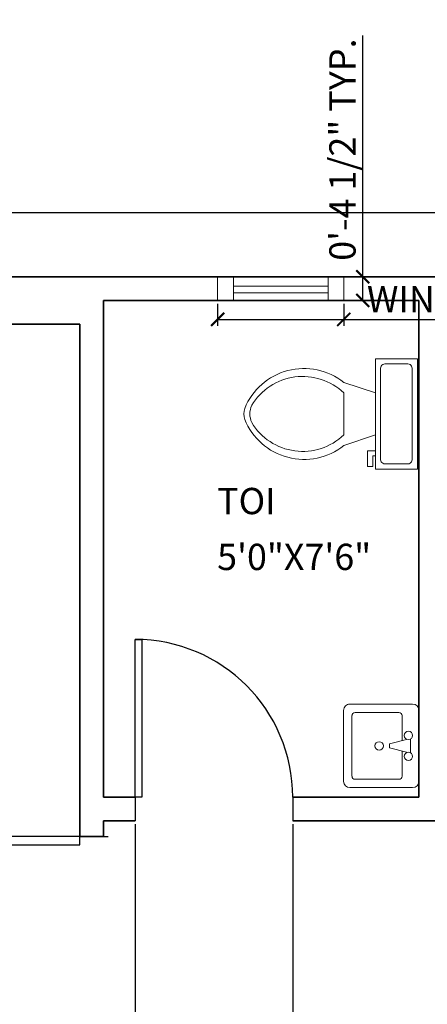
# Model space of a CAD drawing. Units: inches. Extents: x 3283068 to 3284536, y 3240756 to 3241803.
# Tile 12 of 19: x 3283520 to 3283598, y 3241501 to 3241688. Entities that reach past the tile are written whole.
import ezdxf

# ---------------------------------------------------------------- set-up
doc = ezdxf.new("R2010")
doc.units = ezdxf.units.IN
for name, color, linetype, lineweight in [('A-ANNO-DIMS', 2, 'Continuous', 18), ('A-AREA-IDEN', 7, 'Continuous', 18), ('A-FLOR-FIXT', 9, 'Continuous', 18), ('door', 140, 'Continuous', 25), ('wall', 20, 'Continuous', 35), ('window', 100, 'Continuous', 18)]:
    doc.layers.add(name, color=color, linetype=linetype, lineweight=lineweight)
doc.styles.get("Standard").update_dxf_attribs({"font": 'arial.ttf'})
doc.dimstyles.new('ISO-25', dxfattribs={"dimtxt": 5, "dimasz": 2.5, "dimexe": 1.25, "dimexo": 0.625, "dimtad": 1, "dimlunit": 4, "dimtxsty": 'Standard', "dimblk": 'ARCHTICK', "dimcen": 2.5, "dimadec": 0, "dimazin": 0, "dimtfac": 1, "dimtmove": 0, "dimatfit": 3, "dimfxl": 1, "dimarcsym": 0})

# ---------------------------------------------------------------- blocks, each defined once
blk = doc.blocks.new('*U7')
for p, q in [((0, 0), (0, 6)), ((40, 0), (40, 6))]:
    blk.add_line(p, q)
blk.add_lwpolyline([(0, 0), (0, -40), (1.75, -40), (1.75, 0)], close=True)
blk.add_arc((0, 0), 40, 270, 0)
blk = doc.blocks.new('*U4')
for p, q in [((-40, 0), (-40, 6)), ((0, 0), (0, 6))]:
    blk.add_line(p, q)
blk.add_lwpolyline([(0, 0), (0, -40), (-1.75, -40), (-1.75, 0)], close=True)
blk.add_arc((0, 0), 40, 180, 270)
blk = doc.blocks.new('*U22')
for p, q in [((241.3, -152.4), (241.3, -50.8)), ((-254, -215.9), (-203.2, -215.9)), ((-254, -241.3), (-254, -215.9)), ((-203.2, -215.9), (-203.2, -203.2)), ((-177.8, -203.2), (-177.8, -241.3)), ((-101.6, -203.2), (-152.4, -355.6)), ((101.6, -203.2), (152.4, -355.6)), ((-177.8, -241.3), (-254, -241.3)), ((101.6, -355.6), (-101.6, -355.6))]:
    blk.add_line(p, q)
blk.add_lwpolyline([(266.7, -203.2), (266.7, 0), (-266.7, 0), (-266.7, -203.2)], close=True)
for points in [[(215.9, -25.4), (-215.9, -25.4)], [(-241.3, -50.8), (-241.3, -152.4)], [(-215.9, -177.8), (215.9, -177.8)]]:
    blk.add_lwpolyline(points)
for centre, radius, start, end in [((-219.1, -47.6), 22.5, 81.8699, 188.1301), ((219.1, -47.6), 22.5, 351.8699, 98.1301), ((-219.1, -155.6), 22.5, 171.8699, 278.1301), ((219.1, -155.6), 22.5, 261.8699, 8.1301), ((89.4, -548.1), 309.1, 141.4691, 247.9714), ((106.7, -554.2), 287.8, 136.3677, 238.9468), ((-89.4, -548.1), 309.1, 292.0284, 38.5307), ((-106.7, -554.2), 287.8, 301.053, 43.6321), ((0, -708.1), 101.6, 245.7318, 294.2682), ((0, -736.6), 101.6, 254.8605, 285.1395)]:
    blk.add_arc(centre, radius, start, end)
blk = doc.blocks.new('_ArchTick')
at = {"color": 0, "linetype": 'ByBlock', "const_width": 0.15}
blk.add_lwpolyline([(-0.5, -0.5), (0.5, 0.5)], dxfattribs=at)
blk = doc.blocks.new('*D25')
at = {"layer": 'A-ANNO-DIMS', "color": 0, "lineweight": -2, "transparency": 16777216}
for p, q in [((3283339.59, 3241639.73), (3283339.59, 3241652.58)), ((3283339.59, 3241651.33), (3284236.59, 3241651.33)), ((3284236.59, 3241639.73), (3284236.59, 3241652.58))]:
    blk.add_line(p, q, dxfattribs=at)
at = {"layer": 'Defpoints', "color": 0, "transparency": 16777216}
for p in [(3284236.59, 3241651.33), (3283339.59, 3241639.1), (3284236.59, 3241639.1)]:
    blk.add_point(p, dxfattribs=at)
at = {"layer": 'A-ANNO-DIMS', "color": 0, "lineweight": -2, "transparency": 16777216, "xscale": 2.5, "yscale": 2.5, "zscale": 2.5, "rotation": 180}
blk.add_blockref('_ArchTick', (3283339.59, 3241651.33), dxfattribs=at)
at = {"layer": 'A-ANNO-DIMS', "color": 0, "lineweight": -2, "transparency": 16777216, "xscale": 2.5, "yscale": 2.5, "zscale": 2.5}
blk.add_blockref('_ArchTick', (3284236.59, 3241651.33), dxfattribs=at)
at = {"layer": 'A-ANNO-DIMS', "color": 0, "transparency": 16777216, "insert": (3283788.09, 3241654.51), "char_height": 5, "attachment_point": 5}
blk.add_mtext('74\'-9"', dxfattribs=at)
blk = doc.blocks.new('WIN-24IN-4_5IN-WALL')
for p, q in [((0, 4.5), (24, 4.5)), ((0, 0), (0, 4.5)), ((3, 0), (3, 4.5)), ((21, 4.5), (21, 0)), ((24, 4.5), (24, 0)), ((3, 2.73), (21, 2.73)), ((24, 0), (0, 0)), ((3, 1.44), (21, 1.44))]:
    blk.add_line(p, q)
blk = doc.blocks.new('LAVATORY-COMPACT')
for p, q in [((13.12, 15.9), (1.19, 15.9)), ((0, 14.71), (0, 1.19)), ((3.18, 8.94), (3.18, 13.71)), ((3.78, 14.31), (12.12, 14.31)), ((12.72, 13.71), (12.72, 2.19)), ((14.31, 1.19), (14.31, 14.71)), ((1.59, 6.76), (1.59, 9.14)), ((5.56, 8.35), (2.38, 9.14)), ((2.38, 6.76), (5.56, 7.55)), ((5.56, 7.55), (5.56, 8.35)), ((3.18, 2.19), (3.18, 6.96)), ((1.19, 0), (13.12, 0)), ((12.12, 1.59), (3.78, 1.59))]:
    blk.add_line(p, q)
for centre in [(1.99, 9.94), (7.55, 7.95), (1.99, 5.96)]:
    blk.add_circle(centre, 0.795)
for centre, radius, start, end in [((1.19, 14.71), 1.19, 90, 180), ((13.12, 14.71), 1.19, 0, 90), ((3.78, 13.71), 0.596, 90, 180), ((12.12, 13.71), 0.596, 0, 90), ((3.78, 2.19), 0.596, 180, 270), ((12.12, 2.19), 0.596, 270, 0), ((1.19, 1.19), 1.19, 180, 270), ((13.12, 1.19), 1.19, 270, 0)]:
    blk.add_arc(centre, radius, start, end)
blk = doc.blocks.new('*D43')
at = {"layer": 'A-ANNO-DIMS', "color": 0, "lineweight": -2, "transparency": 16777216}
for p, q in [((3283557.81, 3241633.98), (3283557.81, 3241629.75)), ((3283581.81, 3241633.98), (3283581.81, 3241629.75)), ((3283557.81, 3241631), (3283581.81, 3241631)), ((3283581.81, 3241631), (3283648.83, 3241631))]:
    blk.add_line(p, q, dxfattribs=at)
at = {"layer": 'Defpoints', "color": 0, "transparency": 16777216}
for p in [(3283557.81, 3241634.6), (3283581.81, 3241634.6), (3283581.81, 3241631)]:
    blk.add_point(p, dxfattribs=at)
at = {"layer": 'A-ANNO-DIMS', "color": 0, "lineweight": -2, "transparency": 16777216, "xscale": 2.5, "yscale": 2.5, "zscale": 2.5, "rotation": 180}
blk.add_blockref('_ArchTick', (3283557.81, 3241631), dxfattribs=at)
at = {"layer": 'A-ANNO-DIMS', "color": 0, "lineweight": -2, "transparency": 16777216, "xscale": 2.5, "yscale": 2.5, "zscale": 2.5}
blk.add_blockref('_ArchTick', (3283581.81, 3241631), dxfattribs=at)
at = {"layer": 'A-ANNO-DIMS', "color": 0, "transparency": 16777216, "insert": (3283616.57, 3241634.21), "char_height": 5, "attachment_point": 5}
blk.add_mtext('WINDOW 2\'-0" TYP.', dxfattribs=at)
blk = doc.blocks.new('*D44')
at = {"layer": 'A-ANNO-DIMS', "color": 0, "lineweight": -2, "transparency": 16777216}
for p, q in [((3283585.41, 3241639.1), (3283585.41, 3241684.98)), ((3283582.43, 3241639.1), (3283586.66, 3241639.1)), ((3283585.41, 3241634.6), (3283585.41, 3241639.1)), ((3283582.43, 3241634.6), (3283586.66, 3241634.6))]:
    blk.add_line(p, q, dxfattribs=at)
at = {"layer": 'Defpoints', "color": 0, "transparency": 16777216}
for p in [(3283581.81, 3241639.1), (3283585.41, 3241639.1), (3283581.81, 3241634.6)]:
    blk.add_point(p, dxfattribs=at)
at = {"layer": 'A-ANNO-DIMS', "color": 0, "lineweight": -2, "transparency": 16777216, "xscale": 2.5, "yscale": 2.5, "zscale": 2.5}
for p, rotation in [((3283585.41, 3241639.1), 90), ((3283585.41, 3241634.6), 270)]:
    blk.add_blockref('_ArchTick', p, dxfattribs=dict(at, rotation=rotation))
at = {"layer": 'A-ANNO-DIMS', "color": 0, "transparency": 16777216, "insert": (3283582.2, 3241663.29), "char_height": 5, "attachment_point": 5, "rotation": 90}
blk.add_mtext('0\'-4 1/2" TYP.', dxfattribs=at)
blk = doc.blocks.new('*D63')
at = {"layer": 'A-ANNO-DIMS', "color": 0, "lineweight": -2, "transparency": 16777216}
for p, q in [((3283248.09, 3241083.23), (3283248.09, 3241798.08)), ((3284328.09, 3241083.23), (3284328.09, 3241798.08)), ((3283248.09, 3241796.83), (3284328.09, 3241796.83))]:
    blk.add_line(p, q, dxfattribs=at)
at = {"layer": 'Defpoints', "color": 0, "transparency": 16777216}
for p in [(3284328.09, 3241796.83), (3283248.09, 3241082.6), (3284328.09, 3241082.6)]:
    blk.add_point(p, dxfattribs=at)
at = {"layer": 'A-ANNO-DIMS', "color": 0, "lineweight": -2, "transparency": 16777216, "xscale": 2.5, "yscale": 2.5, "zscale": 2.5, "rotation": 180}
blk.add_blockref('_ArchTick', (3283248.09, 3241796.83), dxfattribs=at)
at = {"layer": 'A-ANNO-DIMS', "color": 0, "lineweight": -2, "transparency": 16777216, "xscale": 2.5, "yscale": 2.5, "zscale": 2.5}
blk.add_blockref('_ArchTick', (3284328.09, 3241796.83), dxfattribs=at)
at = {"layer": 'A-ANNO-DIMS', "color": 0, "transparency": 16777216, "insert": (3283788.09, 3241800.01), "char_height": 5, "attachment_point": 5}
blk.add_mtext('90\'-0"', dxfattribs=at)
blk = doc.blocks.new('*D64')
at = {"layer": 'A-ANNO-DIMS', "color": 0, "lineweight": -2, "transparency": 16777216}
for p, q in [((3283542.09, 3241534.98), (3283542.09, 3240759.03)), ((3283572.09, 3241534.98), (3283572.09, 3240759.03)), ((3283542.09, 3240760.28), (3283572.09, 3240760.28))]:
    blk.add_line(p, q, dxfattribs=at)
at = {"layer": 'Defpoints', "color": 0, "transparency": 16777216}
for p in [(3283542.09, 3241535.6), (3283572.09, 3241535.6), (3283572.09, 3240760.28)]:
    blk.add_point(p, dxfattribs=at)
at = {"layer": 'A-ANNO-DIMS', "color": 0, "lineweight": -2, "transparency": 16777216, "xscale": 2.5, "yscale": 2.5, "zscale": 2.5, "rotation": 180}
blk.add_blockref('_ArchTick', (3283542.09, 3240760.28), dxfattribs=at)
at = {"layer": 'A-ANNO-DIMS', "color": 0, "lineweight": -2, "transparency": 16777216, "xscale": 2.5, "yscale": 2.5, "zscale": 2.5}
blk.add_blockref('_ArchTick', (3283572.09, 3240760.28), dxfattribs=at)
at = {"layer": 'A-ANNO-DIMS', "color": 0, "transparency": 16777216, "insert": (3283557.09, 3240763.46), "char_height": 5, "attachment_point": 5}
blk.add_mtext('2\'-6"', dxfattribs=at)

msp = doc.modelspace()

# ---------------------------------------------------------------- linework, layer by layer
at = {"layer": 'door'}
for p, q in [((3283542.089, 3241540.102), (3283542.089, 3241535.602)), ((3283572.089, 3241540.102), (3283572.089, 3241535.602))]:
    msp.add_line(p, q, dxfattribs=at)
at = {"layer": 'wall'}
for p, q in [((3283339.589, 3241639.102), (3284236.589, 3241639.102)), ((3283536.089, 3241634.602), (3283536.089, 3241540.102)), ((3283536.089, 3241634.602), (3283596.089, 3241634.602)), ((3283596.089, 3241634.602), (3283596.089, 3241540.102)), ((3283348.589, 3241630.102), (3283531.589, 3241630.102)), ((3283531.589, 3241630.102), (3283531.589, 3241532.602)), ((3283536.089, 3241540.102), (3283542.089, 3241540.102)), ((3283572.089, 3241540.102), (3283596.089, 3241540.102)), ((3283536.089, 3241535.602), (3283542.089, 3241535.602)), ((3283536.089, 3241535.602), (3283536.089, 3241532.602)), ((3283572.089, 3241535.602), (3283660.589, 3241535.602)), ((3283531.589, 3241532.602), (3283536.089, 3241532.602))]:
    msp.add_line(p, q, dxfattribs=at)

# ---------------------------------------------------------------- block references
at = {"layer": 'A-FLOR-FIXT', "xscale": -0.0393700787401575, "yscale": 0.0393700787401575, "zscale": 0.0393700787401575, "rotation": 270}
msp.add_blockref('*U22', (3283595.816, 3241613.005), dxfattribs=at)
at = {"layer": 'A-FLOR-FIXT', "rotation": 180}
msp.add_blockref('LAVATORY-COMPACT', (3283596.089, 3241557.803), dxfattribs=at)
at = {"layer": 'door'}
for name, p, xscale, yscale, zscale, rotation in [('*U4', (3283542.089, 3241540.102), 0.75, 0.75, 0.75, 180), ('*U7', (3283531.589, 3241532.602), 0.9, 0.9, 0.9, 270)]:
    msp.add_blockref(name, p, dxfattribs=dict(at, xscale=xscale, yscale=yscale, zscale=zscale, rotation=rotation))
at = {"layer": 'window'}
msp.add_blockref('WIN-24IN-4_5IN-WALL', (3283557.806, 3241634.602), dxfattribs=at)

# ---------------------------------------------------------------- texts
at = {"layer": 'A-AREA-IDEN'}
for s, p in [('TOI', (3283557.708, 3241593.934)), ('5\'0"X7\'6"', (3283557.708, 3241583.304))]:
    msp.add_text(s, height=5, dxfattribs=at).set_placement(p)

# ---------------------------------------------------------------- dimensions: what is measured, and where the dimension line sits
at = {"layer": 'A-ANNO-DIMS'}
for base, p1, p2, override, picture, middle in [((3284328.089, 3241796.827), (3283248.089, 3241082.602), (3284328.089, 3241082.602), {"dimdec": 1, "dimlfac": 1, "dimrnd": 0, "dimzin": 1, "dimdsep": 46, "dimlunit": 4, "dimfrac": 2}, '*D63', (3283788.089, 3241800.005)), ((3284236.589, 3241651.334), (3283339.589, 3241639.102), (3284236.589, 3241639.102), {"dimclrd": 0, "dimclre": 0, "dimclrt": 0}, '*D25', (3283788.089, 3241654.512)), ((3283572.089, 3240760.281), (3283542.089, 3241535.602), (3283572.089, 3241535.602), {"dimdec": 1, "dimlfac": 1, "dimrnd": 0, "dimzin": 1, "dimdsep": 46, "dimlunit": 4, "dimfrac": 2}, '*D64', (3283557.089, 3240763.459))]:
    dim = msp.add_linear_dim(base=base, p1=p1, p2=p2, dimstyle='ISO-25', override=override, dxfattribs=at)
    dim.commit()
    dim.dimension.update_dxf_attribs({"geometry": picture, "text_midpoint": middle})
dim = msp.add_linear_dim(base=(3283585.406, 3241639.102), p1=(3283581.806, 3241634.602), p2=(3283581.806, 3241639.102), angle=90, text='<> TYP.', dimstyle='ISO-25', override={"dimdec": 1, "dimlfac": 1, "dimrnd": 0, "dimzin": 1, "dimdsep": 46, "dimlunit": 4, "dimfrac": 2}, dxfattribs=at)
dim.commit()
dim.dimension.update_dxf_attribs({"geometry": '*D44', "text_midpoint": (3283582.195, 3241663.292)})
dim = msp.add_linear_dim(base=(3283581.806, 3241631.002), p1=(3283557.806, 3241634.602), p2=(3283581.806, 3241634.602), text='WINDOW <> TYP.', dimstyle='ISO-25', override={"dimdec": 1, "dimlfac": 1, "dimrnd": 0, "dimzin": 1, "dimdsep": 46, "dimlunit": 4, "dimfrac": 2}, dxfattribs=at)
dim.commit()
dim.dimension.update_dxf_attribs({"geometry": '*D43', "text_midpoint": (3283616.566, 3241634.214)})

doc.saveas('drawing.dxf')
